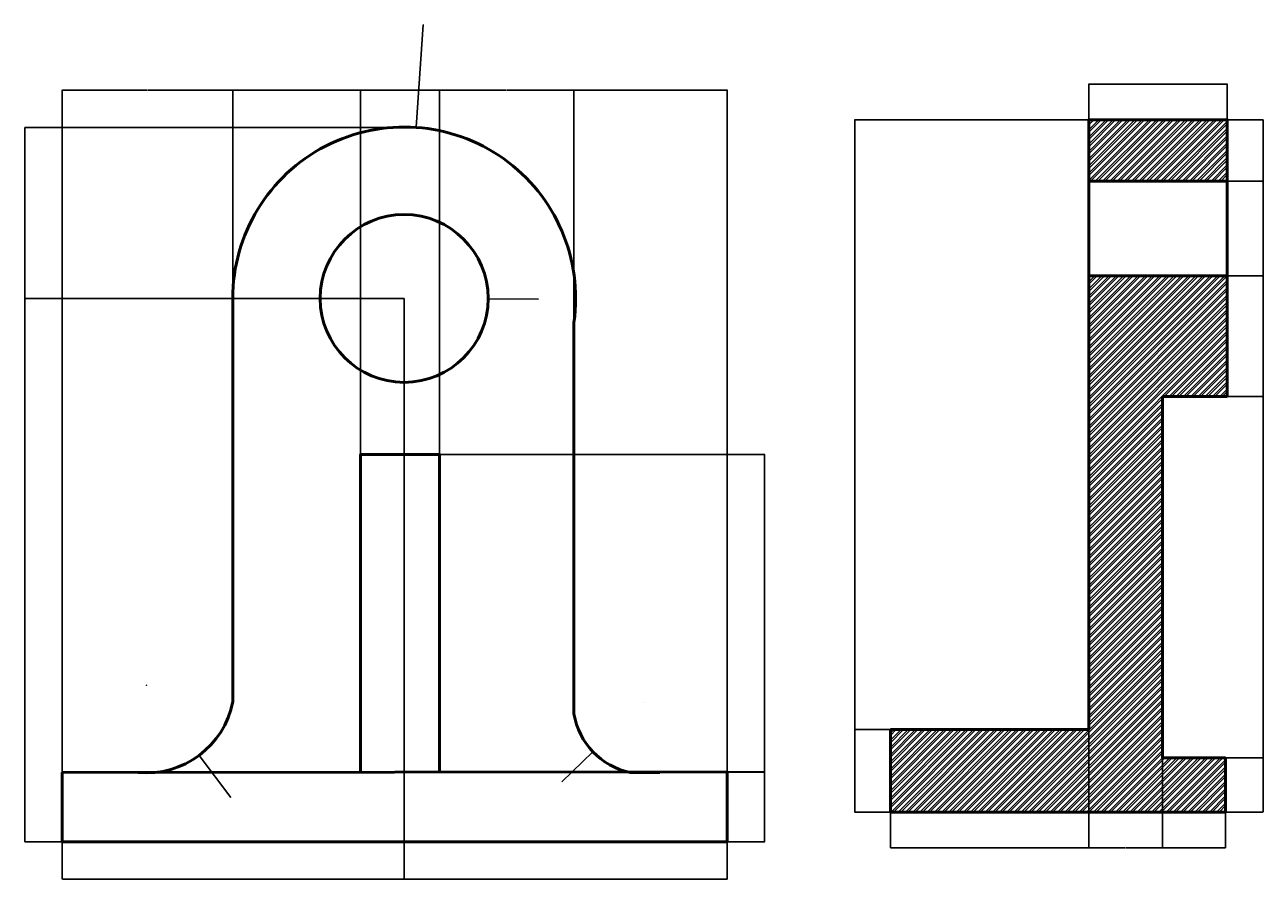
# Model space of a CAD drawing. Units: millimetres. Extents: x 1192 to 5273, y 919 to 2510.
# Tile 1 of 2: x 1192 to 3498, y 919 to 2510. Entities that reach past the tile are written whole.
import ezdxf

# ---------------------------------------------------------------- set-up
doc = ezdxf.new("R2010")
doc.units = ezdxf.units.MM
for name, color, linetype, lineweight in [('M-DIMS', 2, 'Continuous', 18), ('M-HATC', 8, 'Continuous', 18), ('M-OUTL', 7, 'Continuous', 50)]:
    doc.layers.add(name, color=color, linetype=linetype, lineweight=lineweight)
doc.styles.get("Standard").update_dxf_attribs({"font": 'arial.ttf'})
doc.dimstyles.get("Standard").update_dxf_attribs({"dimtxt": 0.18, "dimasz": 0.18, "dimexe": 0.18, "dimexo": 0.0625, "dimgap": 0.09, "dimtad": 0, "dimtih": 1, "dimtoh": 1, "dimdec": 4, "dimzin": 0, "dimdsep": 46, "dimtxsty": 'Standard', "dimcen": 0.09, "dimadec": 0, "dimazin": 0, "dimtfac": 1, "dimtdec": 4, "dimtofl": 0, "dimtmove": 0, "dimatfit": 3, "dimfxl": 1, "dimtolj": 1, "dimtzin": 0, "dimarcsym": 0})

# ---------------------------------------------------------------- blocks, each defined once
blk = doc.blocks.new('*D1')
at = {"layer": 'Defpoints', "color": 0, "transparency": 16777216}
for p in [(1262.3, 988.8), (2500.2, 988.8), (2500.2, 919.3)]:
    blk.add_point(p, dxfattribs=at)
at = {"layer": 'M-DIMS', "color": 0, "lineweight": -2, "transparency": 16777216}
for p, q in [((1262.3, 988.8), (1262.3, 919.1)), ((2500.2, 988.8), (2500.2, 919.1)), ((1262.5, 919.3), (1880.9, 919.3)), ((2500.1, 919.3), (1881.6, 919.3))]:
    blk.add_line(p, q, dxfattribs=at)
at = {"layer": 'M-DIMS', "color": 0, "transparency": 16777216}
for points in [[(1262.5, 919.4), (1262.5, 919.3), (1262.3, 919.3)], [(2500.1, 919.4), (2500.1, 919.3), (2500.2, 919.3)]]:
    blk.add_solid(points, dxfattribs=at)
at = {"layer": 'M-DIMS', "color": 0, "transparency": 16777216, "insert": (1881.3, 919.3), "char_height": 0.18, "attachment_point": 5}
blk.add_mtext('\\A1;1238', dxfattribs=at)
blk = doc.blocks.new('*D2')
at = {"layer": 'Defpoints', "color": 0, "transparency": 16777216}
for p in [(1579.6, 2388.8), (1579.6, 2000.7), (1262.3, 1118)]:
    blk.add_point(p, dxfattribs=at)
at = {"layer": 'M-DIMS', "color": 0, "lineweight": -2, "transparency": 16777216}
for p, q in [((1262.3, 1118.1), (1262.3, 2389)), ((1262.5, 2388.8), (1420.6, 2388.8)), ((1579.4, 2388.8), (1421.3, 2388.8)), ((1579.6, 2000.8), (1579.6, 2389))]:
    blk.add_line(p, q, dxfattribs=at)
at = {"layer": 'M-DIMS', "color": 0, "transparency": 16777216}
for points in [[(1262.5, 2388.8), (1262.5, 2388.8), (1262.3, 2388.8)], [(1579.4, 2388.8), (1579.4, 2388.8), (1579.6, 2388.8)]]:
    blk.add_solid(points, dxfattribs=at)
at = {"layer": 'M-DIMS', "color": 0, "transparency": 16777216, "insert": (1420.9, 2388.8), "char_height": 0.18, "attachment_point": 5}
blk.add_mtext('\\A1;317.2', dxfattribs=at)
blk = doc.blocks.new('*D3')
at = {"layer": 'Defpoints', "color": 0, "transparency": 16777216}
for p in [(1817.6, 2388.8), (1579.6, 2000.7), (1817.6, 1710.1)]:
    blk.add_point(p, dxfattribs=at)
at = {"layer": 'M-DIMS', "color": 0, "lineweight": -2, "transparency": 16777216}
for p, q in [((1579.6, 2000.8), (1579.6, 2389)), ((1579.7, 2388.8), (1698.1, 2388.8)), ((1817.4, 2388.8), (1699, 2388.8)), ((1817.6, 1710.2), (1817.6, 2389))]:
    blk.add_line(p, q, dxfattribs=at)
at = {"layer": 'M-DIMS', "color": 0, "transparency": 16777216}
for points in [[(1579.7, 2388.8), (1579.7, 2388.8), (1579.6, 2388.8)], [(1817.4, 2388.8), (1817.4, 2388.8), (1817.6, 2388.8)]]:
    blk.add_solid(points, dxfattribs=at)
at = {"layer": 'M-DIMS', "color": 0, "transparency": 16777216, "insert": (1698.6, 2388.8), "char_height": 0.18, "attachment_point": 5}
blk.add_mtext('\\A1;238.04', dxfattribs=at)
blk = doc.blocks.new('*D4')
at = {"layer": 'Defpoints', "color": 0, "transparency": 16777216}
for p in [(1964.6, 2388.8), (1817.6, 1710.1), (1964.6, 1710.1)]:
    blk.add_point(p, dxfattribs=at)
at = {"layer": 'M-DIMS', "color": 0, "lineweight": -2, "transparency": 16777216}
for p, q in [((1817.6, 1710.2), (1817.6, 2389)), ((1817.8, 2388.8), (1890.6, 2388.8)), ((1964.4, 2388.8), (1891.5, 2388.8)), ((1964.6, 1710.2), (1964.6, 2389))]:
    blk.add_line(p, q, dxfattribs=at)
at = {"layer": 'M-DIMS', "color": 0, "transparency": 16777216}
for points in [[(1817.8, 2388.8), (1817.8, 2388.8), (1817.6, 2388.8)], [(1964.4, 2388.8), (1964.4, 2388.8), (1964.6, 2388.8)]]:
    blk.add_solid(points, dxfattribs=at)
at = {"layer": 'M-DIMS', "color": 0, "transparency": 16777216, "insert": (1891.1, 2388.8), "char_height": 0.18, "attachment_point": 5}
blk.add_mtext('\\A1;146.98', dxfattribs=at)
blk = doc.blocks.new('*D5')
at = {"layer": 'Defpoints', "color": 0, "transparency": 16777216}
for p in [(2214.8, 2388.8), (2214.8, 1956), (1964.6, 1710.1)]:
    blk.add_point(p, dxfattribs=at)
at = {"layer": 'M-DIMS', "color": 0, "lineweight": -2, "transparency": 16777216}
for p, q in [((1964.6, 1710.2), (1964.6, 2389)), ((1964.8, 2388.8), (2089.2, 2388.8)), ((2214.7, 2388.8), (2090.2, 2388.8)), ((2214.8, 1956), (2214.8, 2389))]:
    blk.add_line(p, q, dxfattribs=at)
at = {"layer": 'M-DIMS', "color": 0, "transparency": 16777216}
for points in [[(1964.8, 2388.8), (1964.8, 2388.8), (1964.6, 2388.8)], [(2214.7, 2388.8), (2214.7, 2388.8), (2214.8, 2388.8)]]:
    blk.add_solid(points, dxfattribs=at)
at = {"layer": 'M-DIMS', "color": 0, "transparency": 16777216, "insert": (2089.7, 2388.8), "char_height": 0.18, "attachment_point": 5}
blk.add_mtext('\\A1;250.27', dxfattribs=at)
blk = doc.blocks.new('*D6')
at = {"layer": 'Defpoints', "color": 0, "transparency": 16777216}
for p in [(2500.2, 2388.8), (2214.8, 1956), (2500.2, 1119.4)]:
    blk.add_point(p, dxfattribs=at)
at = {"layer": 'M-DIMS', "color": 0, "lineweight": -2, "transparency": 16777216}
for p, q in [((2214.8, 1956), (2214.8, 2389)), ((2215, 2388.8), (2357.1, 2388.8)), ((2500.1, 2388.8), (2357.9, 2388.8)), ((2500.2, 1119.4), (2500.2, 2389))]:
    blk.add_line(p, q, dxfattribs=at)
at = {"layer": 'M-DIMS', "color": 0, "transparency": 16777216}
for points in [[(2215, 2388.8), (2215, 2388.8), (2214.8, 2388.8)], [(2500.1, 2388.8), (2500.1, 2388.8), (2500.2, 2388.8)]]:
    blk.add_solid(points, dxfattribs=at)
at = {"layer": 'M-DIMS', "color": 0, "transparency": 16777216, "insert": (2357.5, 2388.8), "char_height": 0.18, "attachment_point": 5}
blk.add_mtext('\\A1;285.4', dxfattribs=at)
blk = doc.blocks.new('*D7')
at = {"layer": 'Defpoints', "color": 0, "transparency": 16777216}
for p in [(2500.2, 1119.4), (2569.7, 1119.4), (2500.2, 988.8)]:
    blk.add_point(p, dxfattribs=at)
at = {"layer": 'M-DIMS', "color": 0, "lineweight": -2, "transparency": 16777216}
for p, q in [((2500.3, 1119.4), (2569.9, 1119.4)), ((2569.7, 1119.2), (2569.7, 1054.3)), ((2569.7, 989), (2569.7, 1053.9)), ((2500.3, 988.8), (2569.9, 988.8))]:
    blk.add_line(p, q, dxfattribs=at)
at = {"layer": 'M-DIMS', "color": 0, "transparency": 16777216}
for points in [[(2569.7, 1119.2), (2569.8, 1119.2), (2569.7, 1119.4)], [(2569.7, 989), (2569.8, 989), (2569.7, 988.8)]]:
    blk.add_solid(points, dxfattribs=at)
at = {"layer": 'M-DIMS', "color": 0, "transparency": 16777216, "insert": (2569.7, 1054.1), "char_height": 0.18, "attachment_point": 5}
blk.add_mtext('\\A1;130.56', dxfattribs=at)
blk = doc.blocks.new('*D8')
at = {"layer": 'Defpoints', "color": 0, "transparency": 16777216}
for p in [(1192.8, 2000.7), (1898.8, 2000.7), (1262.3, 988.8)]:
    blk.add_point(p, dxfattribs=at)
at = {"layer": 'M-DIMS', "color": 0, "lineweight": -2, "transparency": 16777216}
for p, q in [((1898.7, 2000.7), (1192.7, 2000.7)), ((1192.8, 2000.6), (1192.8, 1495)), ((1192.8, 989), (1192.8, 1494.6)), ((1262.3, 988.8), (1192.7, 988.8))]:
    blk.add_line(p, q, dxfattribs=at)
at = {"layer": 'M-DIMS', "color": 0, "transparency": 16777216}
for points in [[(1192.8, 2000.6), (1192.9, 2000.6), (1192.8, 2000.7)], [(1192.8, 989), (1192.9, 989), (1192.8, 988.8)]]:
    blk.add_solid(points, dxfattribs=at)
at = {"layer": 'M-DIMS', "color": 0, "transparency": 16777216, "insert": (1192.8, 1494.8), "char_height": 0.18, "attachment_point": 5}
blk.add_mtext('\\A1;1012', dxfattribs=at)
blk = doc.blocks.new('*D9')
at = {"layer": 'Defpoints', "color": 0, "transparency": 16777216}
for p in [(1192.8, 2319.2), (1921.2, 2319.2), (1262.3, 988.8)]:
    blk.add_point(p, dxfattribs=at)
at = {"layer": 'M-DIMS', "color": 0, "lineweight": -2, "transparency": 16777216}
for p, q in [((1921.2, 2319.2), (1192.7, 2319.2)), ((1192.8, 2319), (1192.8, 1654.2)), ((1192.8, 989), (1192.8, 1653.8)), ((1262.3, 988.8), (1192.7, 988.8))]:
    blk.add_line(p, q, dxfattribs=at)
at = {"layer": 'M-DIMS', "color": 0, "transparency": 16777216}
for points in [[(1192.8, 2319), (1192.9, 2319), (1192.8, 2319.2)], [(1192.8, 989), (1192.9, 989), (1192.8, 988.8)]]:
    blk.add_solid(points, dxfattribs=at)
at = {"layer": 'M-DIMS', "color": 0, "transparency": 16777216, "insert": (1192.8, 1654), "char_height": 0.18, "attachment_point": 5}
blk.add_mtext('\\A1;1330.3', dxfattribs=at)
blk = doc.blocks.new('*D10')
at = {"layer": 'Defpoints', "color": 0, "transparency": 16777216}
for p in [(1898.8, 2000.7), (1262.3, 988.8), (1898.8, 919.3)]:
    blk.add_point(p, dxfattribs=at)
at = {"layer": 'M-DIMS', "color": 0, "lineweight": -2, "transparency": 16777216}
for p, q in [((1898.8, 2000.7), (1898.8, 919.1)), ((1262.3, 988.8), (1262.3, 919.1)), ((1262.5, 919.3), (1580.2, 919.3)), ((1898.6, 919.3), (1581, 919.3))]:
    blk.add_line(p, q, dxfattribs=at)
at = {"layer": 'M-DIMS', "color": 0, "transparency": 16777216}
for points in [[(1262.5, 919.4), (1262.5, 919.3), (1262.3, 919.3)], [(1898.6, 919.4), (1898.6, 919.3), (1898.8, 919.3)]]:
    blk.add_solid(points, dxfattribs=at)
at = {"layer": 'M-DIMS', "color": 0, "transparency": 16777216, "insert": (1580.6, 919.3), "char_height": 0.18, "attachment_point": 5}
blk.add_mtext('\\A1;636.4', dxfattribs=at)
blk = doc.blocks.new('*D11')
at = {"layer": 'Defpoints', "color": 0, "transparency": 16777216}
for p in [(1964.6, 1710.1), (2569.7, 1710.1), (1964.6, 1118.8)]:
    blk.add_point(p, dxfattribs=at)
at = {"layer": 'M-DIMS', "color": 0, "lineweight": -2, "transparency": 16777216}
for p, q in [((1964.6, 1710.1), (2569.9, 1710.1)), ((2569.7, 1710), (2569.7, 1414.6)), ((2569.7, 1119), (2569.7, 1414.3)), ((1964.6, 1118.8), (2569.9, 1118.8))]:
    blk.add_line(p, q, dxfattribs=at)
at = {"layer": 'M-DIMS', "color": 0, "transparency": 16777216}
for points in [[(2569.7, 1710), (2569.8, 1710), (2569.7, 1710.1)], [(2569.7, 1119), (2569.8, 1119), (2569.7, 1118.8)]]:
    blk.add_solid(points, dxfattribs=at)
at = {"layer": 'M-DIMS', "color": 0, "transparency": 16777216, "insert": (2569.7, 1414.5), "char_height": 0.18, "attachment_point": 5}
blk.add_mtext('\\A1;591.4', dxfattribs=at)
blk = doc.blocks.new('*D12')
at = {"layer": 'Defpoints', "color": 0, "transparency": 16777216}
for p in [(2804, 1197.7), (3173.1, 1197.7), (3173.1, 977.8)]:
    blk.add_point(p, dxfattribs=at)
at = {"layer": 'M-DIMS', "color": 0, "lineweight": -2, "transparency": 16777216}
for p, q in [((2804, 1197.6), (2804, 977.6)), ((3173.1, 1197.6), (3173.1, 977.6)), ((2804.2, 977.8), (2988.2, 977.8)), ((3172.9, 977.8), (2988.9, 977.8))]:
    blk.add_line(p, q, dxfattribs=at)
at = {"layer": 'M-DIMS', "color": 0, "transparency": 16777216}
for points in [[(2804.2, 977.8), (2804.2, 977.8), (2804, 977.8)], [(3172.9, 977.8), (3172.9, 977.8), (3173.1, 977.8)]]:
    blk.add_solid(points, dxfattribs=at)
at = {"layer": 'M-DIMS', "color": 0, "transparency": 16777216, "insert": (2988.5, 977.8), "char_height": 0.18, "attachment_point": 5}
blk.add_mtext('\\A1;369.1', dxfattribs=at)
blk = doc.blocks.new('*D13')
at = {"layer": 'Defpoints', "color": 0, "transparency": 16777216}
for p in [(3173.1, 1197.7), (3310.2, 1145.5), (3310.2, 977.8)]:
    blk.add_point(p, dxfattribs=at)
at = {"layer": 'M-DIMS', "color": 0, "lineweight": -2, "transparency": 16777216}
for p, q in [((3173.1, 1197.6), (3173.1, 977.6)), ((3310.2, 1145.4), (3310.2, 977.6)), ((3173.2, 977.8), (3241.2, 977.8)), ((3310.1, 977.8), (3242.1, 977.8))]:
    blk.add_line(p, q, dxfattribs=at)
at = {"layer": 'M-DIMS', "color": 0, "transparency": 16777216}
for points in [[(3173.2, 977.8), (3173.2, 977.8), (3173.1, 977.8)], [(3310.1, 977.8), (3310.1, 977.8), (3310.2, 977.8)]]:
    blk.add_solid(points, dxfattribs=at)
at = {"layer": 'M-DIMS', "color": 0, "transparency": 16777216, "insert": (3241.7, 977.8), "char_height": 0.18, "attachment_point": 5}
blk.add_mtext('\\A1;137.18', dxfattribs=at)
blk = doc.blocks.new('*D14')
at = {"layer": 'Defpoints', "color": 0, "transparency": 16777216}
for p in [(3310.2, 1145.5), (3427.8, 1145.5), (3427.8, 977.8)]:
    blk.add_point(p, dxfattribs=at)
at = {"layer": 'M-DIMS', "color": 0, "lineweight": -2, "transparency": 16777216}
for p, q in [((3310.2, 1145.4), (3310.2, 977.6)), ((3427.8, 1145.4), (3427.8, 977.6)), ((3310.4, 977.8), (3368.6, 977.8)), ((3427.6, 977.8), (3369.5, 977.8))]:
    blk.add_line(p, q, dxfattribs=at)
at = {"layer": 'M-DIMS', "color": 0, "transparency": 16777216}
for points in [[(3310.4, 977.8), (3310.4, 977.8), (3310.2, 977.8)], [(3427.6, 977.8), (3427.6, 977.8), (3427.8, 977.8)]]:
    blk.add_solid(points, dxfattribs=at)
at = {"layer": 'M-DIMS', "color": 0, "transparency": 16777216, "insert": (3369, 977.8), "char_height": 0.18, "attachment_point": 5}
blk.add_mtext('\\A1;117.58', dxfattribs=at)
blk = doc.blocks.new('*D15')
at = {"layer": 'Defpoints', "color": 0, "transparency": 16777216}
for p in [(3173.1, 2333.5), (2737.5, 1197.7), (3173.1, 1197.7)]:
    blk.add_point(p, dxfattribs=at)
at = {"layer": 'M-DIMS', "color": 0, "lineweight": -2, "transparency": 16777216}
for p, q in [((3173, 2333.5), (2737.3, 2333.5)), ((2737.5, 2333.4), (2737.5, 1765.8)), ((2737.5, 1197.9), (2737.5, 1765.4)), ((3173, 1197.7), (2737.3, 1197.7))]:
    blk.add_line(p, q, dxfattribs=at)
at = {"layer": 'M-DIMS', "color": 0, "transparency": 16777216}
for points in [[(2737.5, 2333.4), (2737.5, 2333.4), (2737.5, 2333.5)], [(2737.5, 1197.9), (2737.5, 1197.9), (2737.5, 1197.7)]]:
    blk.add_solid(points, dxfattribs=at)
at = {"layer": 'M-DIMS', "color": 0, "transparency": 16777216, "insert": (2737.5, 1765.6), "char_height": 0.18, "attachment_point": 5}
blk.add_mtext('\\A1;1135.8', dxfattribs=at)
blk = doc.blocks.new('*D16')
at = {"layer": 'Defpoints', "color": 0, "transparency": 16777216}
for p in [(2737.5, 1197.7), (2804, 1197.7), (2804, 1044.3)]:
    blk.add_point(p, dxfattribs=at)
at = {"layer": 'M-DIMS', "color": 0, "lineweight": -2, "transparency": 16777216}
for p, q in [((2803.9, 1197.7), (2737.3, 1197.7)), ((2737.5, 1197.5), (2737.5, 1121.2)), ((2737.5, 1044.5), (2737.5, 1120.8)), ((2803.9, 1044.3), (2737.3, 1044.3))]:
    blk.add_line(p, q, dxfattribs=at)
at = {"layer": 'M-DIMS', "color": 0, "transparency": 16777216}
for points in [[(2737.5, 1197.5), (2737.5, 1197.5), (2737.5, 1197.7)], [(2737.5, 1044.5), (2737.5, 1044.5), (2737.5, 1044.3)]]:
    blk.add_solid(points, dxfattribs=at)
at = {"layer": 'M-DIMS', "color": 0, "transparency": 16777216, "insert": (2737.5, 1121), "char_height": 0.18, "attachment_point": 5}
blk.add_mtext('\\A1;153.4', dxfattribs=at)
blk = doc.blocks.new('*D17')
at = {"layer": 'Defpoints', "color": 0, "transparency": 16777216}
for p in [(2737.5, 2333.5), (3173.1, 2333.5), (2804, 1044.3)]:
    blk.add_point(p, dxfattribs=at)
at = {"layer": 'M-DIMS', "color": 0, "lineweight": -2, "transparency": 16777216}
for p, q in [((3173, 2333.5), (2737.3, 2333.5)), ((2737.5, 2333.4), (2737.5, 1689.1)), ((2737.5, 1044.5), (2737.5, 1688.7)), ((2803.9, 1044.3), (2737.3, 1044.3))]:
    blk.add_line(p, q, dxfattribs=at)
at = {"layer": 'M-DIMS', "color": 0, "transparency": 16777216}
for points in [[(2737.5, 2333.4), (2737.5, 2333.4), (2737.5, 2333.5)], [(2737.5, 1044.5), (2737.5, 1044.5), (2737.5, 1044.3)]]:
    blk.add_solid(points, dxfattribs=at)
at = {"layer": 'M-DIMS', "color": 0, "transparency": 16777216, "insert": (2737.5, 1688.9), "char_height": 0.18, "attachment_point": 5}
blk.add_mtext('\\A1;1289.2', dxfattribs=at)
blk = doc.blocks.new('*D18')
at = {"layer": 'Defpoints', "color": 0, "transparency": 16777216}
for p in [(3431.1, 2400), (3173.1, 2333.5), (3431.1, 2333.5)]:
    blk.add_point(p, dxfattribs=at)
at = {"layer": 'M-DIMS', "color": 0, "lineweight": -2, "transparency": 16777216}
for p, q in [((3173.1, 2333.6), (3173.1, 2400.2)), ((3173.2, 2400), (3301.6, 2400)), ((3430.9, 2400), (3302.5, 2400)), ((3431.1, 2333.6), (3431.1, 2400.2))]:
    blk.add_line(p, q, dxfattribs=at)
at = {"layer": 'M-DIMS', "color": 0, "transparency": 16777216}
for points in [[(3173.2, 2400.1), (3173.2, 2400), (3173.1, 2400)], [(3430.9, 2400.1), (3430.9, 2400), (3431.1, 2400)]]:
    blk.add_solid(points, dxfattribs=at)
at = {"layer": 'M-DIMS', "color": 0, "transparency": 16777216, "insert": (3302.1, 2400), "char_height": 0.18, "attachment_point": 5}
blk.add_mtext('\\A1;258.03', dxfattribs=at)
blk = doc.blocks.new('*D19')
at = {"layer": 'Defpoints', "color": 0, "transparency": 16777216}
for p in [(3427.8, 1145.5), (3497.6, 1145.5), (3427.8, 1044.3)]:
    blk.add_point(p, dxfattribs=at)
at = {"layer": 'M-DIMS', "color": 0, "lineweight": -2, "transparency": 16777216}
for p, q in [((3427.9, 1145.5), (3497.8, 1145.5)), ((3497.6, 1145.3), (3497.6, 1095.1)), ((3497.6, 1044.5), (3497.6, 1094.7)), ((3427.9, 1044.3), (3497.8, 1044.3))]:
    blk.add_line(p, q, dxfattribs=at)
at = {"layer": 'M-DIMS', "color": 0, "transparency": 16777216}
for points in [[(3497.6, 1145.3), (3497.6, 1145.3), (3497.6, 1145.5)], [(3497.6, 1044.5), (3497.6, 1044.5), (3497.6, 1044.3)]]:
    blk.add_solid(points, dxfattribs=at)
at = {"layer": 'M-DIMS', "color": 0, "transparency": 16777216, "insert": (3497.6, 1094.9), "char_height": 0.18, "attachment_point": 5}
blk.add_mtext('\\A1;101.18', dxfattribs=at)
blk = doc.blocks.new('*D20')
at = {"layer": 'Defpoints', "color": 0, "transparency": 16777216}
for p in [(3431.1, 1817.9), (3497.6, 1817.9), (3427.8, 1145.5)]:
    blk.add_point(p, dxfattribs=at)
at = {"layer": 'M-DIMS', "color": 0, "lineweight": -2, "transparency": 16777216}
for p, q in [((3431.2, 1817.9), (3497.8, 1817.9)), ((3497.6, 1817.7), (3497.6, 1481.9)), ((3497.6, 1145.7), (3497.6, 1481.5)), ((3427.9, 1145.5), (3497.8, 1145.5))]:
    blk.add_line(p, q, dxfattribs=at)
at = {"layer": 'M-DIMS', "color": 0, "transparency": 16777216}
for points in [[(3497.6, 1817.7), (3497.6, 1817.7), (3497.6, 1817.9)], [(3497.6, 1145.7), (3497.6, 1145.7), (3497.6, 1145.5)]]:
    blk.add_solid(points, dxfattribs=at)
at = {"layer": 'M-DIMS', "color": 0, "transparency": 16777216, "insert": (3497.6, 1481.7), "char_height": 0.18, "attachment_point": 5}
blk.add_mtext('\\A1;672.4', dxfattribs=at)
blk = doc.blocks.new('*D21')
at = {"layer": 'Defpoints', "color": 0, "transparency": 16777216}
for p in [(3431.1, 2043.1), (3497.6, 2043.1), (3431.1, 1817.9)]:
    blk.add_point(p, dxfattribs=at)
at = {"layer": 'M-DIMS', "color": 0, "lineweight": -2, "transparency": 16777216}
for p, q in [((3431.2, 2043.1), (3497.8, 2043.1)), ((3497.6, 2042.9), (3497.6, 1930.6)), ((3497.6, 1818), (3497.6, 1930.3)), ((3431.2, 1817.9), (3497.8, 1817.9))]:
    blk.add_line(p, q, dxfattribs=at)
at = {"layer": 'M-DIMS', "color": 0, "transparency": 16777216}
for points in [[(3497.6, 2042.9), (3497.6, 2042.9), (3497.6, 2043.1)], [(3497.6, 1818), (3497.6, 1818), (3497.6, 1817.9)]]:
    blk.add_solid(points, dxfattribs=at)
at = {"layer": 'M-DIMS', "color": 0, "transparency": 16777216, "insert": (3497.6, 1930.5), "char_height": 0.18, "attachment_point": 5}
blk.add_mtext('\\A1;225.2', dxfattribs=at)
blk = doc.blocks.new('*D22')
at = {"layer": 'Defpoints', "color": 0, "transparency": 16777216}
for p in [(3431.1, 2219.3), (3497.6, 2219.3), (3431.1, 2043.1)]:
    blk.add_point(p, dxfattribs=at)
at = {"layer": 'M-DIMS', "color": 0, "lineweight": -2, "transparency": 16777216}
for p, q in [((3431.2, 2219.3), (3497.8, 2219.3)), ((3497.6, 2219.1), (3497.6, 2131.4)), ((3497.6, 2043.2), (3497.6, 2131)), ((3431.2, 2043.1), (3497.8, 2043.1))]:
    blk.add_line(p, q, dxfattribs=at)
at = {"layer": 'M-DIMS', "color": 0, "transparency": 16777216}
for points in [[(3497.6, 2219.1), (3497.6, 2219.1), (3497.6, 2219.3)], [(3497.6, 2043.2), (3497.6, 2043.2), (3497.6, 2043.1)]]:
    blk.add_solid(points, dxfattribs=at)
at = {"layer": 'M-DIMS', "color": 0, "transparency": 16777216, "insert": (3497.6, 2131.2), "char_height": 0.18, "attachment_point": 5}
blk.add_mtext('\\A1;176.25', dxfattribs=at)
blk = doc.blocks.new('*D23')
at = {"layer": 'Defpoints', "color": 0, "transparency": 16777216}
for p in [(3431.1, 2333.5), (3497.6, 2333.5), (3431.1, 2219.3)]:
    blk.add_point(p, dxfattribs=at)
at = {"layer": 'M-DIMS', "color": 0, "lineweight": -2, "transparency": 16777216}
for p, q in [((3431.2, 2333.5), (3497.8, 2333.5)), ((3497.6, 2333.4), (3497.6, 2276.6)), ((3497.6, 2219.5), (3497.6, 2276.3)), ((3431.2, 2219.3), (3497.8, 2219.3))]:
    blk.add_line(p, q, dxfattribs=at)
at = {"layer": 'M-DIMS', "color": 0, "transparency": 16777216}
for points in [[(3497.6, 2333.4), (3497.6, 2333.4), (3497.6, 2333.5)], [(3497.6, 2219.5), (3497.6, 2219.5), (3497.6, 2219.3)]]:
    blk.add_solid(points, dxfattribs=at)
at = {"layer": 'M-DIMS', "color": 0, "transparency": 16777216, "insert": (3497.6, 2276.4), "char_height": 0.18, "attachment_point": 5}
blk.add_mtext('\\A1;114.24', dxfattribs=at)
blk = doc.blocks.new('*D36')
at = {"layer": 'Defpoints', "color": 0, "transparency": 16777216}
for p in [(1921, 2319.2), (1898.8, 2000.7)]:
    blk.add_point(p, dxfattribs=at)
at = {"layer": 'M-DIMS', "color": 0, "lineweight": -2, "transparency": 16777216}
for p, q in [((1934.4, 2510.2), (1921, 2319.4)), ((1934.5, 2510.2), (1934.4, 2510.2)), ((1898.7, 2000.7), (1898.9, 2000.7)), ((1898.8, 2000.6), (1898.8, 2000.8))]:
    blk.add_line(p, q, dxfattribs=at)
at = {"layer": 'M-DIMS', "color": 0, "transparency": 16777216}
blk.add_solid([(1921, 2319.4), (1921.1, 2319.4), (1921, 2319.2)], dxfattribs=at)
at = {"layer": 'M-DIMS', "color": 0, "transparency": 16777216, "insert": (1935, 2510.2), "char_height": 0.18, "attachment_point": 5}
blk.add_mtext('\\A1;R319.2', dxfattribs=at)
blk = doc.blocks.new('*D37')
at = {"layer": 'Defpoints', "color": 0, "transparency": 16777216}
for p in [(1742.5, 2001.5), (2055.1, 2000)]:
    blk.add_point(p, dxfattribs=at)
at = {"layer": 'M-DIMS', "color": 0, "lineweight": -2, "transparency": 16777216}
for p, q in [((1898.7, 2000.7), (1898.9, 2000.7)), ((1898.8, 2000.6), (1898.8, 2000.8)), ((2148.8, 1999.6), (2055.2, 2000))]:
    blk.add_line(p, q, dxfattribs=at)
at = {"layer": 'M-DIMS', "color": 0, "transparency": 16777216}
blk.add_solid([(2055.2, 2000), (2055.2, 2000), (2055.1, 2000)], dxfattribs=at)
at = {"layer": 'M-DIMS', "color": 0, "transparency": 16777216, "insert": (2149.3, 1999.6), "char_height": 0.18, "attachment_point": 5}
blk.add_mtext('\\A1;∅312.6', dxfattribs=at)
blk = doc.blocks.new('*D38')
at = {"layer": 'Defpoints', "color": 0, "transparency": 16777216}
for p in [(1419.3, 1280.3), (1517.1, 1149.9)]:
    blk.add_point(p, dxfattribs=at)
at = {"layer": 'M-DIMS', "color": 0, "lineweight": -2, "transparency": 16777216}
for p, q in [((1419.2, 1280.3), (1419.4, 1280.3)), ((1419.3, 1280.2), (1419.3, 1280.4)), ((1575.8, 1071.6), (1517.2, 1149.7)), ((1576, 1071.6), (1575.8, 1071.6))]:
    blk.add_line(p, q, dxfattribs=at)
at = {"layer": 'M-DIMS', "color": 0, "transparency": 16777216}
blk.add_solid([(1517.2, 1149.7), (1517.2, 1149.7), (1517.1, 1149.9)], dxfattribs=at)
at = {"layer": 'M-DIMS', "color": 0, "transparency": 16777216, "insert": (1576.5, 1071.6), "char_height": 0.18, "attachment_point": 5}
blk.add_mtext('\\A1;R163.05', dxfattribs=at)
blk = doc.blocks.new('*D39')
at = {"layer": 'Defpoints', "color": 0, "transparency": 16777216}
for p in [(2346.9, 1249), (2250.3, 1156.3)]:
    blk.add_point(p, dxfattribs=at)
at = {"layer": 'M-DIMS', "color": 0, "lineweight": -2, "transparency": 16777216}
for p, q in [((2346.8, 1249), (2346.9, 1249)), ((2346.9, 1248.9), (2346.9, 1249)), ((2192.4, 1100.7), (2250.2, 1156.2)), ((2192.2, 1100.7), (2192.4, 1100.7))]:
    blk.add_line(p, q, dxfattribs=at)
at = {"layer": 'M-DIMS', "color": 0, "transparency": 16777216}
blk.add_solid([(2250.2, 1156.2), (2250.2, 1156.2), (2250.3, 1156.3)], dxfattribs=at)
at = {"layer": 'M-DIMS', "color": 0, "transparency": 16777216, "insert": (2191.7, 1100.7), "char_height": 0.18, "attachment_point": 5}
blk.add_mtext('\\A1;R133.81', dxfattribs=at)

msp = doc.modelspace()

# ---------------------------------------------------------------- hatches: boundary and pattern name
at = {"layer": 'M-HATC'}
h = msp.add_hatch(dxfattribs=at)
h.set_pattern_fill('ANSI32', color=256)
h.set_pattern_definition([(45, (-120.849, -238.264), (-6.735192, 6.735192), []), (45, (-116.359, -238.264), (-6.735192, 6.735192), [])])
h.paths.add_polyline_path([(3310.247, 1817.853), (3431.096, 1817.853), (3431.096, 1883.131), (3431.096, 2043.062), (3173.067, 2043.062), (3173.067, 1197.712), (2803.987, 1197.712), (2803.987, 1044.309), (3427.83, 1044.309), (3427.83, 1145.49), (3310.247, 1145.49)])
h.paths.add_polyline_path([(3173.067, 2333.549), (3173.067, 2219.312), (3431.096, 2219.312), (3431.096, 2333.549)])

# ---------------------------------------------------------------- linework, layer by layer
at = {"layer": 'M-OUTL'}
for p, q in [((3173.067, 2043.062), (3173.067, 1197.712)), ((3173.067, 2043.062), (3431.096, 2043.062)), ((3431.096, 2043.062), (3431.096, 1883.131)), ((1579.556, 2000.735), (1579.527, 1682.556)), ((2214.842, 1955.958), (2214.842, 1650.959)), ((3431.096, 1883.131), (3431.096, 1817.853)), ((3431.096, 1817.853), (3310.247, 1817.853)), ((3310.247, 1817.853), (3310.247, 1145.49)), ((1579.527, 1682.556), (1579.501, 1383.863)), ((2214.842, 1650.959), (2214.842, 1394.797)), ((1579.501, 1383.863), (1579.489, 1249.935)), ((2214.842, 1394.797), (2214.842, 1227.088)), ((3173.067, 1197.712), (2803.987, 1197.712)), ((2803.987, 1197.712), (2803.987, 1044.309)), ((3310.247, 1145.49), (3427.83, 1145.49)), ((3427.83, 1044.309), (3427.83, 1145.49)), ((1262.343, 1118.018), (2500.231, 1119.379)), ((1262.343, 1118.018), (1262.343, 988.823)), ((2500.231, 1119.379), (2500.231, 988.823)), ((2803.987, 1044.309), (3427.83, 1044.309)), ((1262.343, 988.823), (2500.231, 988.823))]:
    msp.add_line(p, q, dxfattribs=at)
for points in [[(3173.067, 2219.312), (3431.096, 2219.312), (3431.096, 2333.549), (3173.067, 2333.549)], [(3173.067, 2043.062), (3431.096, 2043.062), (3431.096, 2219.312), (3173.067, 2219.312)]]:
    msp.add_lwpolyline(points, close=True, dxfattribs=at)
for points in [[(1817.596, 1118.628), (1817.596, 1710.144), (1964.575, 1710.144), (1964.575, 1118.79)], [(1403.461, 1118.018), (1435.124, 1118.018)], [(2319.251, 1118.018), (2374.465, 1118.018)]]:
    msp.add_lwpolyline(points, dxfattribs=at)
msp.add_circle((1898.777, 2000.735), 156.293, dxfattribs=at)
for centre, radius, start, end in [((1898.777, 2000.735), 319.221, 351.936606, 180.000001), ((1419.293, 1280.295), 163.047, 264.427882, 349.268745), ((2346.858, 1248.953), 133.814, 189.404496, 258.093921)]:
    msp.add_arc(centre, radius, start, end, dxfattribs=at)

# ---------------------------------------------------------------- dimensions: what is measured, and where the dimension line sits
at = {"layer": 'M-DIMS'}
for center, mpoint, override, picture, middle in [((1898.777, 2000.735), (1921.013, 2319.181), {"dimdec": 1, "dimlfac": 1, "dimrnd": 0, "dimzin": 0, "dimdsep": 46, "dimlunit": 2}, '*D36', (1935.013, 2510.248)), ((1419.293, 1280.295), (1517.112, 1149.85), {"dimdec": 2, "dimlfac": 1, "dimrnd": 0, "dimzin": 0, "dimdsep": 46, "dimlunit": 2}, '*D38', (1576.535, 1071.584)), ((2346.858, 1248.953), (2250.311, 1156.298), {"dimdec": 2, "dimlfac": 1, "dimrnd": 0, "dimzin": 0, "dimdsep": 46, "dimlunit": 2}, '*D39', (2191.67, 1100.705))]:
    dim = msp.add_radius_dim(center=center, mpoint=mpoint, dimstyle='Standard', override=override, dxfattribs=at)
    dim.commit()
    dim.dimension.update_dxf_attribs({"geometry": picture, "text_midpoint": middle, "dimtype": 164})
for base, p1, p2, override, picture, middle in [((3431.096, 2400.049), (3173.067, 2333.549), (3431.096, 2333.549), {"dimdec": 2, "dimlfac": 1, "dimrnd": 0, "dimzin": 0, "dimdsep": 46, "dimlunit": 2}, '*D18', (3302.081, 2400.049)), ((1579.556, 2388.788), (1262.343, 1118.018), (1579.556, 2000.735), {"dimdec": 1, "dimlfac": 1, "dimrnd": 0, "dimzin": 0, "dimdsep": 46, "dimlunit": 2}, '*D2', (1420.95, 2388.788)), ((1817.596, 2388.788), (1579.556, 2000.735), (1817.596, 1710.144), {"dimdec": 2, "dimlfac": 1, "dimrnd": 0, "dimzin": 0, "dimdsep": 46, "dimlunit": 2}, '*D3', (1698.576, 2388.788)), ((1964.575, 2388.788), (1817.596, 1710.144), (1964.575, 1710.144), {"dimdec": 2, "dimlfac": 1, "dimrnd": 0, "dimzin": 0, "dimdsep": 46, "dimlunit": 2}, '*D4', (1891.086, 2388.788)), ((2214.842, 2388.788), (1964.575, 1710.144), (2214.842, 1955.958), {"dimdec": 2, "dimlfac": 1, "dimrnd": 0, "dimzin": 0, "dimdsep": 46, "dimlunit": 2}, '*D5', (2089.708, 2388.788)), ((2500.231, 2388.788), (2214.842, 1955.958), (2500.231, 1119.379), {"dimdec": 1, "dimlfac": 1, "dimrnd": 0, "dimzin": 0, "dimdsep": 46, "dimlunit": 2}, '*D6', (2357.536, 2388.788)), ((1898.777, 919.323), (1262.343, 988.823), (1898.777, 2000.735), {"dimdec": 1, "dimlfac": 1, "dimrnd": 0, "dimzin": 0, "dimdsep": 46, "dimlunit": 2}, '*D10', (1580.56, 919.323)), ((3173.067, 977.809), (2803.987, 1197.712), (3173.067, 1197.712), {"dimdec": 1, "dimlfac": 1, "dimrnd": 0, "dimzin": 0, "dimdsep": 46, "dimlunit": 2}, '*D12', (2988.527, 977.809)), ((3310.247, 977.809), (3173.067, 1197.712), (3310.247, 1145.49), {"dimdec": 2, "dimlfac": 1, "dimrnd": 0, "dimzin": 0, "dimdsep": 46, "dimlunit": 2}, '*D13', (3241.657, 977.809)), ((3427.83, 977.809), (3310.247, 1145.49), (3427.83, 1145.49), {"dimdec": 2, "dimlfac": 1, "dimrnd": 0, "dimzin": 0, "dimdsep": 46, "dimlunit": 2}, '*D14', (3369.038, 977.809)), ((2500.231, 919.323), (1262.343, 988.823), (2500.231, 988.823), {"dimdec": 0, "dimlfac": 1, "dimrnd": 0, "dimzin": 0, "dimdsep": 46, "dimlunit": 2}, '*D1', (1881.287, 919.323))]:
    dim = msp.add_linear_dim(base=base, p1=p1, p2=p2, dimstyle='Standard', override=override, dxfattribs=at)
    dim.commit()
    dim.dimension.update_dxf_attribs({"geometry": picture, "text_midpoint": middle})
for base, p1, p2, override, picture, middle in [((2737.487, 1197.712), (3173.067, 2333.549), (3173.067, 1197.712), {"dimdec": 1, "dimlfac": 1, "dimrnd": 0, "dimzin": 0, "dimdsep": 46, "dimlunit": 2}, '*D15', (2737.487, 1765.631)), ((2737.487, 2333.549), (2803.987, 1044.309), (3173.067, 2333.549), {"dimdec": 1, "dimlfac": 1, "dimrnd": 0, "dimzin": 0, "dimdsep": 46, "dimlunit": 2}, '*D17', (2737.487, 1688.929)), ((3497.596, 2333.549), (3431.096, 2219.312), (3431.096, 2333.549), {"dimdec": 2, "dimlfac": 1, "dimrnd": 0, "dimzin": 0, "dimdsep": 46, "dimlunit": 2}, '*D23', (3497.596, 2276.43)), ((1192.843, 2319.166), (1262.343, 988.823), (1921.221, 2319.166), {"dimdec": 1, "dimlfac": 1, "dimrnd": 0, "dimzin": 0, "dimdsep": 46, "dimlunit": 2}, '*D9', (1192.843, 1653.995)), ((3497.596, 2219.312), (3431.096, 2043.062), (3431.096, 2219.312), {"dimdec": 2, "dimlfac": 1, "dimrnd": 0, "dimzin": 0, "dimdsep": 46, "dimlunit": 2}, '*D22', (3497.596, 2131.187)), ((3497.596, 2043.062), (3431.096, 1817.853), (3431.096, 2043.062), {"dimdec": 1, "dimlfac": 1, "dimrnd": 0, "dimzin": 0, "dimdsep": 46, "dimlunit": 2}, '*D21', (3497.596, 1930.457)), ((1192.843, 2000.735), (1262.343, 988.823), (1898.777, 2000.735), {"dimdec": 0, "dimlfac": 1, "dimrnd": 0, "dimzin": 0, "dimdsep": 46, "dimlunit": 2}, '*D8', (1192.843, 1494.779)), ((3497.596, 1817.853), (3427.83, 1145.49), (3431.096, 1817.853), {"dimdec": 1, "dimlfac": 1, "dimrnd": 0, "dimzin": 0, "dimdsep": 46, "dimlunit": 2}, '*D20', (3497.596, 1481.672)), ((2569.731, 1710.144), (1964.575, 1118.79), (1964.575, 1710.144), {"dimdec": 1, "dimlfac": 1, "dimrnd": 0, "dimzin": 0, "dimdsep": 46, "dimlunit": 2}, '*D11', (2569.731, 1414.467)), ((2737.487, 1197.712), (2803.987, 1044.309), (2803.987, 1197.712), {"dimdec": 1, "dimlfac": 1, "dimrnd": 0, "dimzin": 0, "dimdsep": 46, "dimlunit": 2}, '*D16', (2737.487, 1121.011)), ((3497.596, 1145.49), (3427.83, 1044.309), (3427.83, 1145.49), {"dimdec": 2, "dimlfac": 1, "dimrnd": 0, "dimzin": 0, "dimdsep": 46, "dimlunit": 2}, '*D19', (3497.596, 1094.9)), ((2569.731, 1119.379), (2500.231, 988.823), (2500.231, 1119.379), {"dimdec": 2, "dimlfac": 1, "dimrnd": 0, "dimzin": 0, "dimdsep": 46, "dimlunit": 2}, '*D7', (2569.731, 1054.101))]:
    dim = msp.add_linear_dim(base=base, p1=p1, p2=p2, angle=90, dimstyle='Standard', override=override, dxfattribs=at)
    dim.commit()
    dim.dimension.update_dxf_attribs({"geometry": picture, "text_midpoint": middle})
dim = msp.add_diameter_dim_2p(p1=(1742.485, 2001.47), p2=(2055.069, 2000), dimstyle='Standard', override={"dimdec": 1, "dimlfac": 1, "dimrnd": 0, "dimzin": 0, "dimdsep": 46, "dimlunit": 2}, dxfattribs=at)
dim.commit()
dim.dimension.update_dxf_attribs({"geometry": '*D37', "text_midpoint": (2148.843, 1999.558), "dimtype": 163})

doc.saveas('drawing.dxf')
